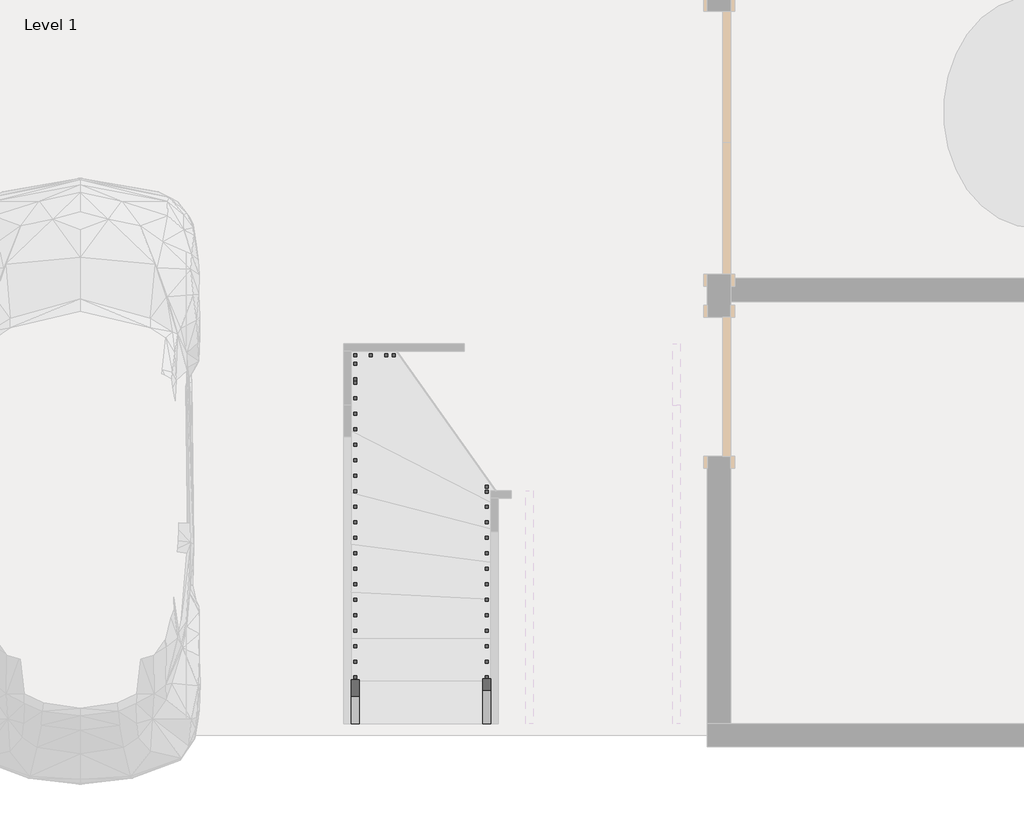
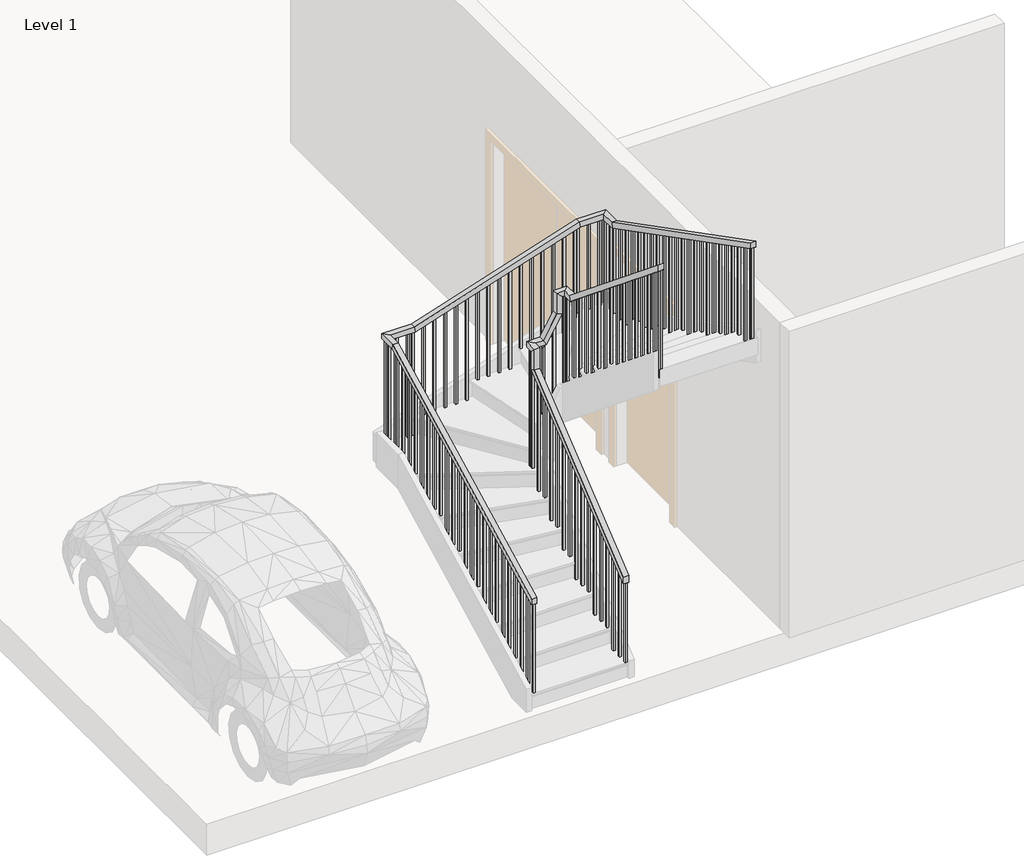
# One storey, part 2 of 4: 2 railings.
"""IFC4 building model written with IfcOpenShell, lengths in millimetres."""

from ifc_helpers import new_model, si_unit, frame, origin, place, context, project, spatial, polyline, outline, extrude, faceted_brep, element, save

model = new_model("IFC4")

# Units and contexts
model_context = context("Model", 3, world=origin())
ifc_project = project(units=[si_unit("LENGTHUNIT", "METRE", prefix="MILLI")], contexts=[model_context])

# Site, building, storey
site = spatial("IfcSite", under=ifc_project)
building = spatial("IfcBuilding", under=site)
storey = spatial("IfcBuildingStorey", under=building, Name="Level 1", Elevation=0.0)

# Railings
placement = place(None, origin())
element("IfcRailing", 1, ObjectType="Handrail - Rectangular", at=placement, inside=storey, context=model_context, shape_type="SolidModel", body=[
    faceted_brep([(-8072.660887, -4607.8089531, 1025.2529681), (-8072.660887, -4607.8089531, 959.7067088), (-8021.860887, -4607.8089531, 959.7067088), (-8021.860887, -4607.8089531, 1025.2529681), (-8072.660887, -3156.2772612, 2208.7848338), (-8072.660887, -3105.4772612, 2184.659247), (-8021.860887, -3105.4772612, 2184.659247), (-8021.860887, -3156.2772612, 2208.7848338), (-8072.660887, -3156.2772612, 2414.6281882), (-8072.660887, -3105.4772612, 2363.8281882), (-8021.860887, -3105.4772612, 2363.8281882), (-8021.860887, -3156.2772612, 2414.6281882), (-8072.660887, -3029.2772612, 2414.6281882), (-8072.660887, -3029.2772612, 2363.8281882), (-8021.860887, -3080.0772612, 2363.8281882), (-8021.860887, -3080.0772612, 2414.6281882), (-7945.660887, -3029.2772612, 2414.6281882), (-7916.5395532, -3029.2772612, 2363.8281882), (-7916.5395532, -3080.0772612, 2363.8281882), (-7945.660887, -3080.0772612, 2414.6281882), (-7818.660887, -3029.2772612, 2631.5051451), (-7767.860887, -3029.2772612, 2617.7256424), (-7767.860887, -3080.0772612, 2617.7256424), (-7818.660887, -3080.0772612, 2631.5051451), (-7818.660887, -3029.2772612, 2837.3484995), (-7767.860887, -3029.2772612, 2786.5484995), (-7767.860887, -3080.0772612, 2786.5484995), (-7818.660887, -3080.0772612, 2837.3484995), (-7691.660887, -3029.2772612, 2837.3484995), (-7691.660887, -3029.2772612, 2786.5484995), (-7742.460887, -3080.0772612, 2786.5484995), (-7742.460887, -3080.0772612, 2837.3484995), (-7691.660887, -3156.2772612, 2837.3484995), (-7691.660887, -3174.3626743, 2786.5484995), (-7742.460887, -3174.3626743, 2786.5484995), (-7742.460887, -3156.2772612, 2837.3484995), (-7691.660887, -4607.8089531, 4020.8803652), (-7742.460887, -4607.8089531, 4020.8803652), (-7742.460887, -4607.8089531, 3955.3341059), (-7691.660887, -4607.8089531, 3955.3341059)], [[[0, 1, 2, 3]], [[1, 0, 4, 5]], [[2, 1, 5, 6]], [[3, 2, 6, 7]], [[0, 3, 7, 4]], [[5, 4, 8, 9]], [[6, 5, 9, 10]], [[7, 6, 10, 11]], [[4, 7, 11, 8]], [[9, 8, 12, 13]], [[10, 9, 13, 14]], [[11, 10, 14, 15]], [[8, 11, 15, 12]], [[13, 12, 16, 17]], [[14, 13, 17, 18]], [[15, 14, 18, 19]], [[12, 15, 19, 16]], [[17, 16, 20, 21]], [[18, 17, 21, 22]], [[19, 18, 22, 23]], [[16, 19, 23, 20]], [[21, 20, 24, 25]], [[22, 21, 25, 26]], [[23, 22, 26, 27]], [[20, 23, 27, 24]], [[25, 24, 28, 29]], [[26, 25, 29, 30]], [[27, 26, 30, 31]], [[24, 27, 31, 28]], [[29, 28, 32, 33]], [[30, 29, 33, 34]], [[31, 30, 34, 35]], [[28, 31, 35, 32]], [[36, 37, 38, 39]], [[33, 32, 36, 39]], [[34, 33, 39, 38]], [[35, 34, 38, 37]], [[32, 35, 37, 36]]]),
    extrude(outline(polyline([(-4517.5696176, 3881.7558784), (-4498.5196176, 3866.2231262), (-4498.5196176, 2878.6666667), (-4517.5696176, 2878.6666667), (-4517.5696176, 3881.7558784)])), frame((-7726.585887, 0.0, 0.0), z_axis=(1.0, 0.0, 0.0), x_axis=(0.0, 1.0, 0.0)), (0.0, 0.0, 1.0), 19.05),
    extrude(outline(polyline([(-4415.9696176, 3798.9145334), (-4396.9196176, 3783.3817813), (-4396.9196176, 2878.6666667), (-4415.9696176, 2878.6666667), (-4415.9696176, 3798.9145334)])), frame((-7726.585887, 0.0, 0.0), z_axis=(1.0, 0.0, 0.0), x_axis=(0.0, 1.0, 0.0)), (0.0, 0.0, 1.0), 19.05),
    extrude(outline(polyline([(-4314.3696176, 3716.0731885), (-4295.3196176, 3700.5404364), (-4295.3196176, 2709.3333333), (-4314.3696176, 2709.3333333), (-4314.3696176, 3716.0731885)])), frame((-7726.585887, 0.0, 0.0), z_axis=(1.0, 0.0, 0.0), x_axis=(0.0, 1.0, 0.0)), (0.0, 0.0, 1.0), 19.05),
    extrude(outline(polyline([(-4212.7696176, 3633.2318436), (-4193.7196176, 3617.6990914), (-4193.7196176, 2709.3333333), (-4212.7696176, 2709.3333333), (-4212.7696176, 3633.2318436)])), frame((-7726.585887, 0.0, 0.0), z_axis=(1.0, 0.0, 0.0), x_axis=(0.0, 1.0, 0.0)), (0.0, 0.0, 1.0), 19.05),
    extrude(outline(polyline([(-4111.1696176, 3550.3904987), (-4092.1196176, 3534.8577465), (-4092.1196176, 2709.3333333), (-4111.1696176, 2709.3333333), (-4111.1696176, 3550.3904987)])), frame((-7726.585887, 0.0, 0.0), z_axis=(1.0, 0.0, 0.0), x_axis=(0.0, 1.0, 0.0)), (0.0, 0.0, 1.0), 19.05),
    extrude(outline(polyline([(-4009.5696176, 3467.5491538), (-3990.5196176, 3452.0164016), (-3990.5196176, 2540.0), (-4009.5696176, 2540.0), (-4009.5696176, 3467.5491538)])), frame((-7726.585887, 0.0, 0.0), z_axis=(1.0, 0.0, 0.0), x_axis=(0.0, 1.0, 0.0)), (0.0, 0.0, 1.0), 19.05),
    extrude(outline(polyline([(-3907.9696176, 3384.7078088), (-3888.9196176, 3369.1750567), (-3888.9196176, 2540.0), (-3907.9696176, 2540.0), (-3907.9696176, 3384.7078088)])), frame((-7726.585887, 0.0, 0.0), z_axis=(1.0, 0.0, 0.0), x_axis=(0.0, 1.0, 0.0)), (0.0, 0.0, 1.0), 19.05),
    extrude(outline(polyline([(-3806.3696176, 3301.8664639), (-3787.3196176, 3286.3337117), (-3787.3196176, 2540.0), (-3806.3696176, 2540.0), (-3806.3696176, 3301.8664639)])), frame((-7726.585887, 0.0, 0.0), z_axis=(1.0, 0.0, 0.0), x_axis=(0.0, 1.0, 0.0)), (0.0, 0.0, 1.0), 19.05),
    extrude(outline(polyline([(-3704.7696176, 3219.025119), (-3685.7196176, 3203.4923668), (-3685.7196176, 2370.6666667), (-3704.7696176, 2370.6666667), (-3704.7696176, 3219.025119)])), frame((-7726.585887, 0.0, 0.0), z_axis=(1.0, 0.0, 0.0), x_axis=(0.0, 1.0, 0.0)), (0.0, 0.0, 1.0), 19.05),
    extrude(outline(polyline([(-3603.1696176, 3136.1837741), (-3584.1196176, 3120.6510219), (-3584.1196176, 2370.6666667), (-3603.1696176, 2370.6666667), (-3603.1696176, 3136.1837741)])), frame((-7726.585887, 0.0, 0.0), z_axis=(1.0, 0.0, 0.0), x_axis=(0.0, 1.0, 0.0)), (0.0, 0.0, 1.0), 19.05),
    extrude(outline(polyline([(-3501.5696176, 3053.3424291), (-3482.5196176, 3037.809677), (-3482.5196176, 2201.3333333), (-3501.5696176, 2201.3333333), (-3501.5696176, 3053.3424291)])), frame((-7726.585887, 0.0, 0.0), z_axis=(1.0, 0.0, 0.0), x_axis=(0.0, 1.0, 0.0)), (0.0, 0.0, 1.0), 19.05),
    extrude(outline(polyline([(-3399.9696176, 2970.5010842), (-3380.9196176, 2954.9683321), (-3380.9196176, 2201.3333333), (-3399.9696176, 2201.3333333), (-3399.9696176, 2970.5010842)])), frame((-7726.585887, 0.0, 0.0), z_axis=(1.0, 0.0, 0.0), x_axis=(0.0, 1.0, 0.0)), (0.0, 0.0, 1.0), 19.05),
    extrude(outline(polyline([(-3298.3696176, 2887.6597393), (-3279.3196176, 2872.1269871), (-3279.3196176, 2032.0), (-3298.3696176, 2032.0), (-3298.3696176, 2887.6597393)])), frame((-7726.585887, 0.0, 0.0), z_axis=(1.0, 0.0, 0.0), x_axis=(0.0, 1.0, 0.0)), (0.0, 0.0, 1.0), 19.05),
    extrude(outline(polyline([(-3196.7696176, 2804.8183944), (-3177.7196176, 2789.2856422), (-3177.7196176, 2032.0), (-3196.7696176, 2032.0), (-3196.7696176, 2804.8183944)])), frame((-7726.585887, 0.0, 0.0), z_axis=(1.0, 0.0, 0.0), x_axis=(0.0, 1.0, 0.0)), (0.0, 0.0, 1.0), 19.05),
    extrude(outline(polyline([(2529.115018, -7819.7499833), (2496.5834745, -7838.7999833), (1524.0, -7838.7999833), (1524.0, -7819.7499833), (2529.115018, -7819.7499833)])), frame((0.0, -3064.2022612, 0.0), z_axis=(0.0, 1.0, 0.0), x_axis=(0.0, 0.0, 1.0)), (0.0, 0.0, 1.0), 19.05),
    extrude(outline(polyline([(2355.6134525, -7921.3499833), (2323.0819089, -7940.3999833), (1524.0, -7940.3999833), (1524.0, -7921.3499833), (2355.6134525, -7921.3499833)])), frame((0.0, -3064.2022612, 0.0), z_axis=(0.0, 1.0, 0.0), x_axis=(0.0, 0.0, 1.0)), (0.0, 0.0, 1.0), 19.05),
    extrude(outline(polyline([(-3194.9339531, 2111.7191617), (-3175.8839531, 2127.2519138), (-3175.8839531, 1016.0), (-3194.9339531, 1016.0), (-3194.9339531, 2111.7191617)])), frame((-8056.785887, 0.0, 0.0), z_axis=(1.0, 0.0, 0.0), x_axis=(0.0, 1.0, 0.0)), (0.0, 0.0, 1.0), 19.05),
    extrude(outline(polyline([(-3296.5339531, 2028.8778167), (-3277.4839531, 2044.4105689), (-3277.4839531, 1016.0), (-3296.5339531, 1016.0), (-3296.5339531, 2028.8778167)])), frame((-8056.785887, 0.0, 0.0), z_axis=(1.0, 0.0, 0.0), x_axis=(0.0, 1.0, 0.0)), (0.0, 0.0, 1.0), 19.05),
    extrude(outline(polyline([(-3398.1339531, 1946.0364718), (-3379.0839531, 1961.569224), (-3379.0839531, 846.6666667), (-3398.1339531, 846.6666667), (-3398.1339531, 1946.0364718)])), frame((-8056.785887, 0.0, 0.0), z_axis=(1.0, 0.0, 0.0), x_axis=(0.0, 1.0, 0.0)), (0.0, 0.0, 1.0), 19.05),
    extrude(outline(polyline([(-3499.7339531, 1863.1951269), (-3480.6839531, 1878.7278791), (-3480.6839531, 846.6666667), (-3499.7339531, 846.6666667), (-3499.7339531, 1863.1951269)])), frame((-8056.785887, 0.0, 0.0), z_axis=(1.0, 0.0, 0.0), x_axis=(0.0, 1.0, 0.0)), (0.0, 0.0, 1.0), 19.05),
    extrude(outline(polyline([(-3601.3339531, 1780.353782), (-3582.2839531, 1795.8865341), (-3582.2839531, 677.3333333), (-3601.3339531, 677.3333333), (-3601.3339531, 1780.353782)])), frame((-8056.785887, 0.0, 0.0), z_axis=(1.0, 0.0, 0.0), x_axis=(0.0, 1.0, 0.0)), (0.0, 0.0, 1.0), 19.05),
    extrude(outline(polyline([(-3702.9339531, 1697.5124371), (-3683.8839531, 1713.0451892), (-3683.8839531, 677.3333333), (-3702.9339531, 677.3333333), (-3702.9339531, 1697.5124371)])), frame((-8056.785887, 0.0, 0.0), z_axis=(1.0, 0.0, 0.0), x_axis=(0.0, 1.0, 0.0)), (0.0, 0.0, 1.0), 19.05),
    extrude(outline(polyline([(-3804.5339531, 1614.6710921), (-3785.4839531, 1630.2038443), (-3785.4839531, 508.0), (-3804.5339531, 508.0), (-3804.5339531, 1614.6710921)])), frame((-8056.785887, 0.0, 0.0), z_axis=(1.0, 0.0, 0.0), x_axis=(0.0, 1.0, 0.0)), (0.0, 0.0, 1.0), 19.05),
    extrude(outline(polyline([(-3906.1339531, 1531.8297472), (-3887.0839531, 1547.3624994), (-3887.0839531, 508.0), (-3906.1339531, 508.0), (-3906.1339531, 1531.8297472)])), frame((-8056.785887, 0.0, 0.0), z_axis=(1.0, 0.0, 0.0), x_axis=(0.0, 1.0, 0.0)), (0.0, 0.0, 1.0), 19.05),
    extrude(outline(polyline([(-4007.7339531, 1448.9884023), (-3988.6839531, 1464.5211545), (-3988.6839531, 508.0), (-4007.7339531, 508.0), (-4007.7339531, 1448.9884023)])), frame((-8056.785887, 0.0, 0.0), z_axis=(1.0, 0.0, 0.0), x_axis=(0.0, 1.0, 0.0)), (0.0, 0.0, 1.0), 19.05),
    extrude(outline(polyline([(-4109.3339531, 1366.1470574), (-4090.2839531, 1381.6798095), (-4090.2839531, 338.6666667), (-4109.3339531, 338.6666667), (-4109.3339531, 1366.1470574)])), frame((-8056.785887, 0.0, 0.0), z_axis=(1.0, 0.0, 0.0), x_axis=(0.0, 1.0, 0.0)), (0.0, 0.0, 1.0), 19.05),
    extrude(outline(polyline([(-4210.9339531, 1283.3057124), (-4191.8839531, 1298.8384646), (-4191.8839531, 338.6666667), (-4210.9339531, 338.6666667), (-4210.9339531, 1283.3057124)])), frame((-8056.785887, 0.0, 0.0), z_axis=(1.0, 0.0, 0.0), x_axis=(0.0, 1.0, 0.0)), (0.0, 0.0, 1.0), 19.05),
    extrude(outline(polyline([(-4312.5339531, 1200.4643675), (-4293.4839531, 1215.9971197), (-4293.4839531, 338.6666667), (-4312.5339531, 338.6666667), (-4312.5339531, 1200.4643675)])), frame((-8056.785887, 0.0, 0.0), z_axis=(1.0, 0.0, 0.0), x_axis=(0.0, 1.0, 0.0)), (0.0, 0.0, 1.0), 19.05),
    extrude(outline(polyline([(-4414.1339531, 1117.6230226), (-4395.0839531, 1133.1557748), (-4395.0839531, 169.3333333), (-4414.1339531, 169.3333333), (-4414.1339531, 1117.6230226)])), frame((-8056.785887, 0.0, 0.0), z_axis=(1.0, 0.0, 0.0), x_axis=(0.0, 1.0, 0.0)), (0.0, 0.0, 1.0), 19.05),
    extrude(outline(polyline([(-4515.7339531, 1034.7816777), (-4496.6839531, 1050.3144298), (-4496.6839531, 169.3333333), (-4515.7339531, 169.3333333), (-4515.7339531, 1034.7816777)])), frame((-8056.785887, 0.0, 0.0), z_axis=(1.0, 0.0, 0.0), x_axis=(0.0, 1.0, 0.0)), (0.0, 0.0, 1.0), 19.05),
    extrude(outline(polyline([(-7726.585887, -3076.1196176), (-7707.535887, -3076.1196176), (-7707.535887, -3095.1696176), (-7726.585887, -3095.1696176), (-7726.585887, -3076.1196176)])), frame((0.0, 0.0, 1862.6666667), z_axis=(0.0, 0.0, 1.0), x_axis=(1.0, 0.0, 0.0)), (0.0, 0.0, 1.0), 923.8818329),
    extrude(outline(polyline([(-7726.585887, -3064.2022612), (-7726.585887, -3045.1522612), (-7707.535887, -3045.1522612), (-7707.535887, -3064.2022612), (-7726.585887, -3064.2022612)])), frame((0.0, 0.0, 1862.6666667), z_axis=(0.0, 0.0, 1.0), x_axis=(1.0, 0.0, 0.0)), (0.0, 0.0, 1.0), 923.8818329),
    extrude(outline(polyline([(-7741.3717908, -3064.2022612), (-7741.3717908, -3045.1522612), (-7722.3217908, -3045.1522612), (-7722.3217908, -3064.2022612), (-7741.3717908, -3064.2022612)])), frame((0.0, 0.0, 1693.3333333), z_axis=(0.0, 0.0, 1.0), x_axis=(1.0, 0.0, 0.0)), (0.0, 0.0, 1.0), 1093.2151662),
    extrude(outline(polyline([(-8041.9999833, -3064.2022612), (-8041.9999833, -3045.1522612), (-8022.9499833, -3045.1522612), (-8022.9499833, -3064.2022612), (-8041.9999833, -3064.2022612)])), frame((0.0, 0.0, 1354.6666667), z_axis=(0.0, 0.0, 1.0), x_axis=(1.0, 0.0, 0.0)), (0.0, 0.0, 1.0), 1009.1615215),
    extrude(outline(polyline([(-8037.735887, -3064.2022612), (-8056.785887, -3064.2022612), (-8056.785887, -3045.1522612), (-8037.735887, -3045.1522612), (-8037.735887, -3064.2022612)])), frame((0.0, 0.0, 1185.3333333), z_axis=(0.0, 0.0, 1.0), x_axis=(1.0, 0.0, 0.0)), (0.0, 0.0, 1.0), 1178.4948549),
    extrude(outline(polyline([(-8037.735887, -3095.1696176), (-8056.785887, -3095.1696176), (-8056.785887, -3076.1196176), (-8037.735887, -3076.1196176), (-8037.735887, -3095.1696176)])), frame((0.0, 0.0, 1185.3333333), z_axis=(0.0, 0.0, 1.0), x_axis=(1.0, 0.0, 0.0)), (0.0, 0.0, 1.0), 1178.4948549),
    extrude(outline(polyline([(-4607.8089531, 3955.3341059), (-4588.7589531, 3939.8013537), (-4588.7589531, 2878.6666667), (-4607.8089531, 2878.6666667), (-4607.8089531, 3955.3341059)])), frame((-7726.585887, 0.0, 0.0), z_axis=(1.0, 0.0, 0.0), x_axis=(0.0, 1.0, 0.0)), (0.0, 0.0, 1.0), 19.05),
    extrude(outline(polyline([(-4607.8089531, 959.7067088), (-4588.7589531, 975.239461), (-4588.7589531, 169.3333333), (-4607.8089531, 169.3333333), (-4607.8089531, 959.7067088)])), frame((-8056.785887, 0.0, 0.0), z_axis=(1.0, 0.0, 0.0), x_axis=(0.0, 1.0, 0.0)), (0.0, 0.0, 1.0), 19.05),
])
element("IfcRailing", 2, ObjectType="Handrail - Rectangular", at=placement, inside=storey, context=model_context, shape_type="SolidModel", body=[
    faceted_brep([(-8936.260887, -4607.8089531, 1109.0771751), (-8936.260887, -4607.8089531, 1051.9280057), (-8885.460887, -4607.8089531, 1051.9280057), (-8885.460887, -4607.8089531, 1109.0771751), (-8936.260887, -2347.8270966, 2273.7644996), (-8936.260887, -2335.5070453, 2222.9644996), (-8885.460887, -2335.5070453, 2222.9644996), (-8885.460887, -2347.8270966, 2273.7644996), (-8936.260887, -2165.6772612, 2273.7644996), (-8936.260887, -2165.6772612, 2222.9644996), (-8885.460887, -2216.4772612, 2222.9644996), (-8885.460887, -2216.4772612, 2273.7644996), (-8659.1069344, -2165.6772612, 2273.7644996), (-8651.1563583, -2165.6772612, 2222.9644996), (-8651.1563583, -2216.4772612, 2222.9644996), (-8659.1069344, -2216.4772612, 2273.7644996), (-7105.2148396, -2165.6772612, 2772.3688337), (-7097.2642635, -2165.6772612, 2721.5688337), (-7097.2642635, -2216.4772612, 2721.5688337), (-7105.2148396, -2216.4772612, 2772.3688337), (-6828.060887, -2165.6772612, 2772.3688337), (-6828.060887, -2165.6772612, 2721.5688337), (-6878.860887, -2216.4772612, 2721.5688337), (-6878.860887, -2216.4772612, 2772.3688337), (-6828.060887, -2347.8270966, 2772.3688337), (-6828.060887, -2360.1471479, 2721.5688337), (-6878.860887, -2360.1471479, 2721.5688337), (-6878.860887, -2347.8270966, 2772.3688337), (-6828.060887, -4607.8089531, 3937.0561582), (-6878.860887, -4607.8089531, 3937.0561582), (-6878.860887, -4607.8089531, 3879.9069889), (-6828.060887, -4607.8089531, 3879.9069889)], [[[0, 1, 2, 3]], [[1, 0, 4, 5]], [[2, 1, 5, 6]], [[3, 2, 6, 7]], [[0, 3, 7, 4]], [[5, 4, 8, 9]], [[6, 5, 9, 10]], [[7, 6, 10, 11]], [[4, 7, 11, 8]], [[9, 8, 12, 13]], [[10, 9, 13, 14]], [[11, 10, 14, 15]], [[8, 11, 15, 12]], [[13, 12, 16, 17]], [[14, 13, 17, 18]], [[15, 14, 18, 19]], [[12, 15, 19, 16]], [[17, 16, 20, 21]], [[18, 17, 21, 22]], [[19, 18, 22, 23]], [[16, 19, 23, 20]], [[21, 20, 24, 25]], [[22, 21, 25, 26]], [[23, 22, 26, 27]], [[20, 23, 27, 24]], [[28, 29, 30, 31]], [[25, 24, 28, 31]], [[26, 25, 31, 30]], [[27, 26, 30, 29]], [[24, 27, 29, 28]]]),
    extrude(outline(polyline([(-4573.5020966, 3862.2268642), (-4573.5020966, 2878.6666667), (-4592.5520966, 2878.6666667), (-4592.5520966, 3872.0443296), (-4573.5020966, 3862.2268642)])), frame((-6862.985887, 0.0, 0.0), z_axis=(1.0, 0.0, 0.0), x_axis=(0.0, 1.0, 0.0)), (0.0, 0.0, 1.0), 19.05),
    extrude(outline(polyline([(-4471.9020966, 3809.8670491), (-4471.9020966, 2878.6666667), (-4490.9520966, 2878.6666667), (-4490.9520966, 3819.6845145), (-4471.9020966, 3809.8670491)])), frame((-6862.985887, 0.0, 0.0), z_axis=(1.0, 0.0, 0.0), x_axis=(0.0, 1.0, 0.0)), (0.0, 0.0, 1.0), 19.05),
    extrude(outline(polyline([(-4370.3020966, 3757.507234), (-4370.3020966, 2878.6666667), (-4389.3520966, 2878.6666667), (-4389.3520966, 3767.3246993), (-4370.3020966, 3757.507234)])), frame((-6862.985887, 0.0, 0.0), z_axis=(1.0, 0.0, 0.0), x_axis=(0.0, 1.0, 0.0)), (0.0, 0.0, 1.0), 19.05),
    extrude(outline(polyline([(-4268.7020966, 3705.1474189), (-4268.7020966, 2709.3333333), (-4287.7520966, 2709.3333333), (-4287.7520966, 3714.9648842), (-4268.7020966, 3705.1474189)])), frame((-6862.985887, 0.0, 0.0), z_axis=(1.0, 0.0, 0.0), x_axis=(0.0, 1.0, 0.0)), (0.0, 0.0, 1.0), 19.05),
    extrude(outline(polyline([(-4167.1020966, 3652.7876038), (-4167.1020966, 2709.3333333), (-4186.1520966, 2709.3333333), (-4186.1520966, 3662.6050691), (-4167.1020966, 3652.7876038)])), frame((-6862.985887, 0.0, 0.0), z_axis=(1.0, 0.0, 0.0), x_axis=(0.0, 1.0, 0.0)), (0.0, 0.0, 1.0), 19.05),
    extrude(outline(polyline([(-4065.5020966, 3600.4277887), (-4065.5020966, 2709.3333333), (-4084.5520966, 2709.3333333), (-4084.5520966, 3610.245254), (-4065.5020966, 3600.4277887)])), frame((-6862.985887, 0.0, 0.0), z_axis=(1.0, 0.0, 0.0), x_axis=(0.0, 1.0, 0.0)), (0.0, 0.0, 1.0), 19.05),
    extrude(outline(polyline([(-3963.9020966, 3548.0679735), (-3963.9020966, 2540.0), (-3982.9520966, 2540.0), (-3982.9520966, 3557.8854389), (-3963.9020966, 3548.0679735)])), frame((-6862.985887, 0.0, 0.0), z_axis=(1.0, 0.0, 0.0), x_axis=(0.0, 1.0, 0.0)), (0.0, 0.0, 1.0), 19.05),
    extrude(outline(polyline([(-3862.3020966, 3495.7081584), (-3862.3020966, 2540.0), (-3881.3520966, 2540.0), (-3881.3520966, 3505.5256238), (-3862.3020966, 3495.7081584)])), frame((-6862.985887, 0.0, 0.0), z_axis=(1.0, 0.0, 0.0), x_axis=(0.0, 1.0, 0.0)), (0.0, 0.0, 1.0), 19.05),
    extrude(outline(polyline([(-3760.7020966, 3443.3483433), (-3760.7020966, 2540.0), (-3779.7520966, 2540.0), (-3779.7520966, 3453.1658086), (-3760.7020966, 3443.3483433)])), frame((-6862.985887, 0.0, 0.0), z_axis=(1.0, 0.0, 0.0), x_axis=(0.0, 1.0, 0.0)), (0.0, 0.0, 1.0), 19.05),
    extrude(outline(polyline([(-3659.1020966, 3390.9885282), (-3659.1020966, 2370.6666667), (-3678.1520966, 2370.6666667), (-3678.1520966, 3400.8059935), (-3659.1020966, 3390.9885282)])), frame((-6862.985887, 0.0, 0.0), z_axis=(1.0, 0.0, 0.0), x_axis=(0.0, 1.0, 0.0)), (0.0, 0.0, 1.0), 19.05),
    extrude(outline(polyline([(-3557.5020966, 3338.6287131), (-3557.5020966, 2370.6666667), (-3576.5520966, 2370.6666667), (-3576.5520966, 3348.4461784), (-3557.5020966, 3338.6287131)])), frame((-6862.985887, 0.0, 0.0), z_axis=(1.0, 0.0, 0.0), x_axis=(0.0, 1.0, 0.0)), (0.0, 0.0, 1.0), 19.05),
    extrude(outline(polyline([(-3455.9020966, 3286.268898), (-3455.9020966, 2370.6666667), (-3474.9520966, 2370.6666667), (-3474.9520966, 3296.0863633), (-3455.9020966, 3286.268898)])), frame((-6862.985887, 0.0, 0.0), z_axis=(1.0, 0.0, 0.0), x_axis=(0.0, 1.0, 0.0)), (0.0, 0.0, 1.0), 19.05),
    extrude(outline(polyline([(-3354.3020966, 3233.9090828), (-3354.3020966, 2201.3333333), (-3373.3520966, 2201.3333333), (-3373.3520966, 3243.7265482), (-3354.3020966, 3233.9090828)])), frame((-6862.985887, 0.0, 0.0), z_axis=(1.0, 0.0, 0.0), x_axis=(0.0, 1.0, 0.0)), (0.0, 0.0, 1.0), 19.05),
    extrude(outline(polyline([(-3252.7020966, 3181.5492677), (-3252.7020966, 2201.3333333), (-3271.7520966, 2201.3333333), (-3271.7520966, 3191.3667331), (-3252.7020966, 3181.5492677)])), frame((-6862.985887, 0.0, 0.0), z_axis=(1.0, 0.0, 0.0), x_axis=(0.0, 1.0, 0.0)), (0.0, 0.0, 1.0), 19.05),
    extrude(outline(polyline([(-3151.1020966, 3129.1894526), (-3151.1020966, 2201.3333333), (-3170.1520966, 2201.3333333), (-3170.1520966, 3139.0069179), (-3151.1020966, 3129.1894526)])), frame((-6862.985887, 0.0, 0.0), z_axis=(1.0, 0.0, 0.0), x_axis=(0.0, 1.0, 0.0)), (0.0, 0.0, 1.0), 19.05),
    extrude(outline(polyline([(-3049.5020966, 3076.8296375), (-3049.5020966, 2032.0), (-3068.5520966, 2032.0), (-3068.5520966, 3086.6471028), (-3049.5020966, 3076.8296375)])), frame((-6862.985887, 0.0, 0.0), z_axis=(1.0, 0.0, 0.0), x_axis=(0.0, 1.0, 0.0)), (0.0, 0.0, 1.0), 19.05),
    extrude(outline(polyline([(-2947.9020966, 3024.4698224), (-2947.9020966, 2032.0), (-2966.9520966, 2032.0), (-2966.9520966, 3034.2872877), (-2947.9020966, 3024.4698224)])), frame((-6862.985887, 0.0, 0.0), z_axis=(1.0, 0.0, 0.0), x_axis=(0.0, 1.0, 0.0)), (0.0, 0.0, 1.0), 19.05),
    extrude(outline(polyline([(-2846.3020966, 2972.1100073), (-2846.3020966, 2032.0), (-2865.3520966, 2032.0), (-2865.3520966, 2981.9274726), (-2846.3020966, 2972.1100073)])), frame((-6862.985887, 0.0, 0.0), z_axis=(1.0, 0.0, 0.0), x_axis=(0.0, 1.0, 0.0)), (0.0, 0.0, 1.0), 19.05),
    extrude(outline(polyline([(-2744.7020966, 2919.7501921), (-2744.7020966, 2032.0), (-2763.7520966, 2032.0), (-2763.7520966, 2929.5676575), (-2744.7020966, 2919.7501921)])), frame((-6862.985887, 0.0, 0.0), z_axis=(1.0, 0.0, 0.0), x_axis=(0.0, 1.0, 0.0)), (0.0, 0.0, 1.0), 19.05),
    extrude(outline(polyline([(-2643.1020966, 2867.390377), (-2643.1020966, 1862.6666667), (-2662.1520966, 1862.6666667), (-2662.1520966, 2877.2078424), (-2643.1020966, 2867.390377)])), frame((-6862.985887, 0.0, 0.0), z_axis=(1.0, 0.0, 0.0), x_axis=(0.0, 1.0, 0.0)), (0.0, 0.0, 1.0), 19.05),
    extrude(outline(polyline([(-2541.5020966, 2815.0305619), (-2541.5020966, 1862.6666667), (-2560.5520966, 1862.6666667), (-2560.5520966, 2824.8480272), (-2541.5020966, 2815.0305619)])), frame((-6862.985887, 0.0, 0.0), z_axis=(1.0, 0.0, 0.0), x_axis=(0.0, 1.0, 0.0)), (0.0, 0.0, 1.0), 19.05),
    extrude(outline(polyline([(-2439.9020966, 2762.6707468), (-2439.9020966, 1862.6666667), (-2458.9520966, 1862.6666667), (-2458.9520966, 2772.4882121), (-2439.9020966, 2762.6707468)])), frame((-6862.985887, 0.0, 0.0), z_axis=(1.0, 0.0, 0.0), x_axis=(0.0, 1.0, 0.0)), (0.0, 0.0, 1.0), 19.05),
    extrude(outline(polyline([(-6843.935887, -2283.1522612), (-6843.935887, -2302.2022612), (-6862.985887, -2302.2022612), (-6862.985887, -2283.1522612), (-6843.935887, -2283.1522612)])), frame((0.0, 0.0, 1862.6666667), z_axis=(0.0, 0.0, 1.0), x_axis=(1.0, 0.0, 0.0)), (0.0, 0.0, 1.0), 858.902167),
    extrude(outline(polyline([(-6911.5398396, -2181.5522612), (-6892.4898396, -2181.5522612), (-6892.4898396, -2200.6022612), (-6911.5398396, -2200.6022612), (-6911.5398396, -2181.5522612)])), frame((0.0, 0.0, 1862.6666667), z_axis=(0.0, 0.0, 1.0), x_axis=(1.0, 0.0, 0.0)), (0.0, 0.0, 1.0), 858.902167),
    extrude(outline(polyline([(-7013.1398396, -2181.5522612), (-6994.0898396, -2181.5522612), (-6994.0898396, -2200.6022612), (-7013.1398396, -2200.6022612), (-7013.1398396, -2181.5522612)])), frame((0.0, 0.0, 1862.6666667), z_axis=(0.0, 0.0, 1.0), x_axis=(1.0, 0.0, 0.0)), (0.0, 0.0, 1.0), 858.902167),
    extrude(outline(polyline([(2706.3697564, -7144.6319344), (1693.3333333, -7144.6319344), (1693.3333333, -7125.5819344), (2712.4824155, -7125.5819344), (2706.3697564, -7144.6319344)])), frame((0.0, -2200.6022612, 0.0), z_axis=(0.0, 1.0, 0.0), x_axis=(0.0, 0.0, 1.0)), (0.0, 0.0, 1.0), 19.05),
    extrude(outline(polyline([(2673.7689082, -7246.2319344), (1693.3333333, -7246.2319344), (1693.3333333, -7227.1819344), (2679.8815673, -7227.1819344), (2673.7689082, -7246.2319344)])), frame((0.0, -2200.6022612, 0.0), z_axis=(0.0, 1.0, 0.0), x_axis=(0.0, 0.0, 1.0)), (0.0, 0.0, 1.0), 19.05),
    extrude(outline(polyline([(2641.16806, -7347.8319344), (1693.3333333, -7347.8319344), (1693.3333333, -7328.7819344), (2647.280719, -7328.7819344), (2641.16806, -7347.8319344)])), frame((0.0, -2200.6022612, 0.0), z_axis=(0.0, 1.0, 0.0), x_axis=(0.0, 0.0, 1.0)), (0.0, 0.0, 1.0), 19.05),
    extrude(outline(polyline([(2608.5672118, -7449.4319344), (1693.3333333, -7449.4319344), (1693.3333333, -7430.3819344), (2614.6798708, -7430.3819344), (2608.5672118, -7449.4319344)])), frame((0.0, -2200.6022612, 0.0), z_axis=(0.0, 1.0, 0.0), x_axis=(0.0, 0.0, 1.0)), (0.0, 0.0, 1.0), 19.05),
    extrude(outline(polyline([(2575.9663635, -7551.0319344), (1693.3333333, -7551.0319344), (1693.3333333, -7531.9819344), (2582.0790226, -7531.9819344), (2575.9663635, -7551.0319344)])), frame((0.0, -2200.6022612, 0.0), z_axis=(0.0, 1.0, 0.0), x_axis=(0.0, 0.0, 1.0)), (0.0, 0.0, 1.0), 19.05),
    extrude(outline(polyline([(2543.3655153, -7652.6319344), (1693.3333333, -7652.6319344), (1693.3333333, -7633.5819344), (2549.4781744, -7633.5819344), (2543.3655153, -7652.6319344)])), frame((0.0, -2200.6022612, 0.0), z_axis=(0.0, 1.0, 0.0), x_axis=(0.0, 0.0, 1.0)), (0.0, 0.0, 1.0), 19.05),
    extrude(outline(polyline([(2510.7646671, -7754.2319344), (1524.0, -7754.2319344), (1524.0, -7735.1819344), (2516.8773261, -7735.1819344), (2510.7646671, -7754.2319344)])), frame((0.0, -2200.6022612, 0.0), z_axis=(0.0, 1.0, 0.0), x_axis=(0.0, 0.0, 1.0)), (0.0, 0.0, 1.0), 19.05),
    extrude(outline(polyline([(2478.1638189, -7855.8319344), (1524.0, -7855.8319344), (1524.0, -7836.7819344), (2484.2764779, -7836.7819344), (2478.1638189, -7855.8319344)])), frame((0.0, -2200.6022612, 0.0), z_axis=(0.0, 1.0, 0.0), x_axis=(0.0, 0.0, 1.0)), (0.0, 0.0, 1.0), 19.05),
    extrude(outline(polyline([(2445.5629706, -7957.4319344), (1524.0, -7957.4319344), (1524.0, -7938.3819344), (2451.6756297, -7938.3819344), (2445.5629706, -7957.4319344)])), frame((0.0, -2200.6022612, 0.0), z_axis=(0.0, 1.0, 0.0), x_axis=(0.0, 0.0, 1.0)), (0.0, 0.0, 1.0), 19.05),
    extrude(outline(polyline([(2412.9621224, -8059.0319344), (1524.0, -8059.0319344), (1524.0, -8039.9819344), (2419.0747814, -8039.9819344), (2412.9621224, -8059.0319344)])), frame((0.0, -2200.6022612, 0.0), z_axis=(0.0, 1.0, 0.0), x_axis=(0.0, 0.0, 1.0)), (0.0, 0.0, 1.0), 19.05),
    extrude(outline(polyline([(2380.3612742, -8160.6319344), (1354.6666667, -8160.6319344), (1354.6666667, -8141.5819344), (2386.4739332, -8141.5819344), (2380.3612742, -8160.6319344)])), frame((0.0, -2200.6022612, 0.0), z_axis=(0.0, 1.0, 0.0), x_axis=(0.0, 0.0, 1.0)), (0.0, 0.0, 1.0), 19.05),
    extrude(outline(polyline([(2347.7604259, -8262.2319344), (1354.6666667, -8262.2319344), (1354.6666667, -8243.1819344), (2353.873085, -8243.1819344), (2347.7604259, -8262.2319344)])), frame((0.0, -2200.6022612, 0.0), z_axis=(0.0, 1.0, 0.0), x_axis=(0.0, 0.0, 1.0)), (0.0, 0.0, 1.0), 19.05),
    extrude(outline(polyline([(2315.1595777, -8363.8319344), (1354.6666667, -8363.8319344), (1354.6666667, -8344.7819344), (2321.2722368, -8344.7819344), (2315.1595777, -8363.8319344)])), frame((0.0, -2200.6022612, 0.0), z_axis=(0.0, 1.0, 0.0), x_axis=(0.0, 0.0, 1.0)), (0.0, 0.0, 1.0), 19.05),
    extrude(outline(polyline([(2282.5587295, -8465.4319344), (1354.6666667, -8465.4319344), (1354.6666667, -8446.3819344), (2288.6713885, -8446.3819344), (2282.5587295, -8465.4319344)])), frame((0.0, -2200.6022612, 0.0), z_axis=(0.0, 1.0, 0.0), x_axis=(0.0, 0.0, 1.0)), (0.0, 0.0, 1.0), 19.05),
    extrude(outline(polyline([(2249.9578813, -8567.0319344), (1354.6666667, -8567.0319344), (1354.6666667, -8547.9819344), (2256.0705403, -8547.9819344), (2249.9578813, -8567.0319344)])), frame((0.0, -2200.6022612, 0.0), z_axis=(0.0, 1.0, 0.0), x_axis=(0.0, 0.0, 1.0)), (0.0, 0.0, 1.0), 19.05),
    extrude(outline(polyline([(-8717.185887, -2181.5522612), (-8698.135887, -2181.5522612), (-8698.135887, -2200.6022612), (-8717.185887, -2200.6022612), (-8717.185887, -2181.5522612)])), frame((0.0, 0.0, 1185.3333333), z_axis=(0.0, 0.0, 1.0), x_axis=(1.0, 0.0, 0.0)), (0.0, 0.0, 1.0), 1037.6311663),
    extrude(outline(polyline([(-8818.785887, -2181.5522612), (-8799.735887, -2181.5522612), (-8799.735887, -2200.6022612), (-8818.785887, -2200.6022612), (-8818.785887, -2181.5522612)])), frame((0.0, 0.0, 1185.3333333), z_axis=(0.0, 0.0, 1.0), x_axis=(1.0, 0.0, 0.0)), (0.0, 0.0, 1.0), 1037.6311663),
    extrude(outline(polyline([(-8920.385887, -2255.7520966), (-8920.385887, -2236.7020966), (-8901.335887, -2236.7020966), (-8901.335887, -2255.7520966), (-8920.385887, -2255.7520966)])), frame((0.0, 0.0, 1185.3333333), z_axis=(0.0, 0.0, 1.0), x_axis=(1.0, 0.0, 0.0)), (0.0, 0.0, 1.0), 1037.6311663),
    extrude(outline(polyline([(-2363.0839531, 2208.752671), (-2363.0839531, 1185.3333333), (-2382.1339531, 1185.3333333), (-2382.1339531, 2198.9352056), (-2363.0839531, 2208.752671)])), frame((-8920.385887, 0.0, 0.0), z_axis=(1.0, 0.0, 0.0), x_axis=(0.0, 1.0, 0.0)), (0.0, 0.0, 1.0), 19.05),
    extrude(outline(polyline([(-2464.6839531, 2156.3928558), (-2464.6839531, 1185.3333333), (-2483.7339531, 1185.3333333), (-2483.7339531, 2146.5753905), (-2464.6839531, 2156.3928558)])), frame((-8920.385887, 0.0, 0.0), z_axis=(1.0, 0.0, 0.0), x_axis=(0.0, 1.0, 0.0)), (0.0, 0.0, 1.0), 19.05),
    extrude(outline(polyline([(-2566.2839531, 2104.0330407), (-2566.2839531, 1185.3333333), (-2585.3339531, 1185.3333333), (-2585.3339531, 2094.2155754), (-2566.2839531, 2104.0330407)])), frame((-8920.385887, 0.0, 0.0), z_axis=(1.0, 0.0, 0.0), x_axis=(0.0, 1.0, 0.0)), (0.0, 0.0, 1.0), 19.05),
    extrude(outline(polyline([(-2667.8839531, 2051.6732256), (-2667.8839531, 1185.3333333), (-2686.9339531, 1185.3333333), (-2686.9339531, 2041.8557603), (-2667.8839531, 2051.6732256)])), frame((-8920.385887, 0.0, 0.0), z_axis=(1.0, 0.0, 0.0), x_axis=(0.0, 1.0, 0.0)), (0.0, 0.0, 1.0), 19.05),
    extrude(outline(polyline([(-2769.4839531, 1999.3134105), (-2769.4839531, 1016.0), (-2788.5339531, 1016.0), (-2788.5339531, 1989.4959452), (-2769.4839531, 1999.3134105)])), frame((-8920.385887, 0.0, 0.0), z_axis=(1.0, 0.0, 0.0), x_axis=(0.0, 1.0, 0.0)), (0.0, 0.0, 1.0), 19.05),
    extrude(outline(polyline([(-2871.0839531, 1946.9535954), (-2871.0839531, 1016.0), (-2890.1339531, 1016.0), (-2890.1339531, 1937.13613), (-2871.0839531, 1946.9535954)])), frame((-8920.385887, 0.0, 0.0), z_axis=(1.0, 0.0, 0.0), x_axis=(0.0, 1.0, 0.0)), (0.0, 0.0, 1.0), 19.05),
    extrude(outline(polyline([(-2972.6839531, 1894.5937803), (-2972.6839531, 1016.0), (-2991.7339531, 1016.0), (-2991.7339531, 1884.7763149), (-2972.6839531, 1894.5937803)])), frame((-8920.385887, 0.0, 0.0), z_axis=(1.0, 0.0, 0.0), x_axis=(0.0, 1.0, 0.0)), (0.0, 0.0, 1.0), 19.05),
    extrude(outline(polyline([(-3074.2839531, 1842.2339651), (-3074.2839531, 1016.0), (-3093.3339531, 1016.0), (-3093.3339531, 1832.4164998), (-3074.2839531, 1842.2339651)])), frame((-8920.385887, 0.0, 0.0), z_axis=(1.0, 0.0, 0.0), x_axis=(0.0, 1.0, 0.0)), (0.0, 0.0, 1.0), 19.05),
    extrude(outline(polyline([(-3175.8839531, 1789.87415), (-3175.8839531, 846.6666667), (-3194.9339531, 846.6666667), (-3194.9339531, 1780.0566847), (-3175.8839531, 1789.87415)])), frame((-8920.385887, 0.0, 0.0), z_axis=(1.0, 0.0, 0.0), x_axis=(0.0, 1.0, 0.0)), (0.0, 0.0, 1.0), 19.05),
    extrude(outline(polyline([(-3277.4839531, 1737.5143349), (-3277.4839531, 846.6666667), (-3296.5339531, 846.6666667), (-3296.5339531, 1727.6968696), (-3277.4839531, 1737.5143349)])), frame((-8920.385887, 0.0, 0.0), z_axis=(1.0, 0.0, 0.0), x_axis=(0.0, 1.0, 0.0)), (0.0, 0.0, 1.0), 19.05),
    extrude(outline(polyline([(-3379.0839531, 1685.1545198), (-3379.0839531, 846.6666667), (-3398.1339531, 846.6666667), (-3398.1339531, 1675.3370545), (-3379.0839531, 1685.1545198)])), frame((-8920.385887, 0.0, 0.0), z_axis=(1.0, 0.0, 0.0), x_axis=(0.0, 1.0, 0.0)), (0.0, 0.0, 1.0), 19.05),
    extrude(outline(polyline([(-3480.6839531, 1632.7947047), (-3480.6839531, 677.3333333), (-3499.7339531, 677.3333333), (-3499.7339531, 1622.9772393), (-3480.6839531, 1632.7947047)])), frame((-8920.385887, 0.0, 0.0), z_axis=(1.0, 0.0, 0.0), x_axis=(0.0, 1.0, 0.0)), (0.0, 0.0, 1.0), 19.05),
    extrude(outline(polyline([(-3582.2839531, 1580.4348896), (-3582.2839531, 677.3333333), (-3601.3339531, 677.3333333), (-3601.3339531, 1570.6174242), (-3582.2839531, 1580.4348896)])), frame((-8920.385887, 0.0, 0.0), z_axis=(1.0, 0.0, 0.0), x_axis=(0.0, 1.0, 0.0)), (0.0, 0.0, 1.0), 19.05),
    extrude(outline(polyline([(-3683.8839531, 1528.0750744), (-3683.8839531, 677.3333333), (-3702.9339531, 677.3333333), (-3702.9339531, 1518.2576091), (-3683.8839531, 1528.0750744)])), frame((-8920.385887, 0.0, 0.0), z_axis=(1.0, 0.0, 0.0), x_axis=(0.0, 1.0, 0.0)), (0.0, 0.0, 1.0), 19.05),
    extrude(outline(polyline([(-3785.4839531, 1475.7152593), (-3785.4839531, 508.0), (-3804.5339531, 508.0), (-3804.5339531, 1465.897794), (-3785.4839531, 1475.7152593)])), frame((-8920.385887, 0.0, 0.0), z_axis=(1.0, 0.0, 0.0), x_axis=(0.0, 1.0, 0.0)), (0.0, 0.0, 1.0), 19.05),
    extrude(outline(polyline([(-3887.0839531, 1423.3554442), (-3887.0839531, 508.0), (-3906.1339531, 508.0), (-3906.1339531, 1413.5379789), (-3887.0839531, 1423.3554442)])), frame((-8920.385887, 0.0, 0.0), z_axis=(1.0, 0.0, 0.0), x_axis=(0.0, 1.0, 0.0)), (0.0, 0.0, 1.0), 19.05),
    extrude(outline(polyline([(-3988.6839531, 1370.9956291), (-3988.6839531, 508.0), (-4007.7339531, 508.0), (-4007.7339531, 1361.1781638), (-3988.6839531, 1370.9956291)])), frame((-8920.385887, 0.0, 0.0), z_axis=(1.0, 0.0, 0.0), x_axis=(0.0, 1.0, 0.0)), (0.0, 0.0, 1.0), 19.05),
    extrude(outline(polyline([(-4090.2839531, 1318.635814), (-4090.2839531, 338.6666667), (-4109.3339531, 338.6666667), (-4109.3339531, 1308.8183486), (-4090.2839531, 1318.635814)])), frame((-8920.385887, 0.0, 0.0), z_axis=(1.0, 0.0, 0.0), x_axis=(0.0, 1.0, 0.0)), (0.0, 0.0, 1.0), 19.05),
    extrude(outline(polyline([(-4191.8839531, 1266.2759989), (-4191.8839531, 338.6666667), (-4210.9339531, 338.6666667), (-4210.9339531, 1256.4585335), (-4191.8839531, 1266.2759989)])), frame((-8920.385887, 0.0, 0.0), z_axis=(1.0, 0.0, 0.0), x_axis=(0.0, 1.0, 0.0)), (0.0, 0.0, 1.0), 19.05),
    extrude(outline(polyline([(-4293.4839531, 1213.9161837), (-4293.4839531, 338.6666667), (-4312.5339531, 338.6666667), (-4312.5339531, 1204.0987184), (-4293.4839531, 1213.9161837)])), frame((-8920.385887, 0.0, 0.0), z_axis=(1.0, 0.0, 0.0), x_axis=(0.0, 1.0, 0.0)), (0.0, 0.0, 1.0), 19.05),
    extrude(outline(polyline([(-4395.0839531, 1161.5563686), (-4395.0839531, 169.3333333), (-4414.1339531, 169.3333333), (-4414.1339531, 1151.7389033), (-4395.0839531, 1161.5563686)])), frame((-8920.385887, 0.0, 0.0), z_axis=(1.0, 0.0, 0.0), x_axis=(0.0, 1.0, 0.0)), (0.0, 0.0, 1.0), 19.05),
    extrude(outline(polyline([(-4496.6839531, 1109.1965535), (-4496.6839531, 169.3333333), (-4515.7339531, 169.3333333), (-4515.7339531, 1099.3790882), (-4496.6839531, 1109.1965535)])), frame((-8920.385887, 0.0, 0.0), z_axis=(1.0, 0.0, 0.0), x_axis=(0.0, 1.0, 0.0)), (0.0, 0.0, 1.0), 19.05),
    extrude(outline(polyline([(-6843.935887, -2338.3020966), (-6843.935887, -2357.3520966), (-6862.985887, -2357.3520966), (-6862.985887, -2338.3020966), (-6843.935887, -2338.3020966)])), frame((0.0, 0.0, 1862.6666667), z_axis=(0.0, 0.0, 1.0), x_axis=(1.0, 0.0, 0.0)), (0.0, 0.0, 1.0), 858.902167),
    extrude(outline(polyline([(-6862.985887, -2181.5522612), (-6843.935887, -2181.5522612), (-6843.935887, -2200.6022612), (-6862.985887, -2200.6022612), (-6862.985887, -2181.5522612)])), frame((0.0, 0.0, 1862.6666667), z_axis=(0.0, 0.0, 1.0), x_axis=(1.0, 0.0, 0.0)), (0.0, 0.0, 1.0), 858.902167),
    extrude(outline(polyline([(2715.9613671, -7114.7398396), (1862.6666667, -7114.7398396), (1862.6666667, -7095.6898396), (2722.0740262, -7095.6898396), (2715.9613671, -7114.7398396)])), frame((0.0, -2200.6022612, 0.0), z_axis=(0.0, 1.0, 0.0), x_axis=(0.0, 0.0, 1.0)), (0.0, 0.0, 1.0), 19.05),
    extrude(outline(polyline([(-8668.6319344, -2181.5522612), (-8649.5819344, -2181.5522612), (-8649.5819344, -2200.6022612), (-8668.6319344, -2200.6022612), (-8668.6319344, -2181.5522612)])), frame((0.0, 0.0, 1185.3333333), z_axis=(0.0, 0.0, 1.0), x_axis=(1.0, 0.0, 0.0)), (0.0, 0.0, 1.0), 1037.6311663),
    extrude(outline(polyline([(-8920.385887, -2200.6022612), (-8920.385887, -2181.5522612), (-8901.335887, -2181.5522612), (-8901.335887, -2200.6022612), (-8920.385887, -2200.6022612)])), frame((0.0, 0.0, 1185.3333333), z_axis=(0.0, 0.0, 1.0), x_axis=(1.0, 0.0, 0.0)), (0.0, 0.0, 1.0), 1037.6311663),
    extrude(outline(polyline([(-2338.3020966, 2221.5240629), (-2338.3020966, 1185.3333333), (-2357.3520966, 1185.3333333), (-2357.3520966, 2211.7065976), (-2338.3020966, 2221.5240629)])), frame((-8920.385887, 0.0, 0.0), z_axis=(1.0, 0.0, 0.0), x_axis=(0.0, 1.0, 0.0)), (0.0, 0.0, 1.0), 19.05),
    extrude(outline(polyline([(-4588.7589531, 3870.0895235), (-4588.7589531, 2878.6666667), (-4607.8089531, 2878.6666667), (-4607.8089531, 3879.9069889), (-4588.7589531, 3870.0895235)])), frame((-6862.985887, 0.0, 0.0), z_axis=(1.0, 0.0, 0.0), x_axis=(0.0, 1.0, 0.0)), (0.0, 0.0, 1.0), 19.05),
    extrude(outline(polyline([(-4588.7589531, 1061.7454711), (-4588.7589531, 169.3333333), (-4607.8089531, 169.3333333), (-4607.8089531, 1051.9280057), (-4588.7589531, 1061.7454711)])), frame((-8920.385887, 0.0, 0.0), z_axis=(1.0, 0.0, 0.0), x_axis=(0.0, 1.0, 0.0)), (0.0, 0.0, 1.0), 19.05),
])

save(model, "model.ifc")

# Revit data of these elements
# Type "Handrail - Rectangular"
#   Assembly Code = "C2010400"
#   built-in parameter 1008612 = 0.0416667 (stored number, unit not read)
#   built-in parameter 1008611 = 0.0416667 (stored number, unit not read)
#   built-in parameter 1008609 = 0.333333 (stored number, unit not read)
#   built-in parameter 1008604 = 0.166667 (stored number, unit not read)
#   built-in parameter 1008603 = 0.166667 (stored number, unit not read)
#   Railing Height = 3' - 0"
#   built-in parameter 1008630 = 2
#   built-in parameter 1008610 = 2
#   built-in parameter 1008618 = Baluster - Square : 3/4"
# Elements 1, 2 (IfcRailing, "Handrail - Rectangular")
#   Phase Created = New Construction
